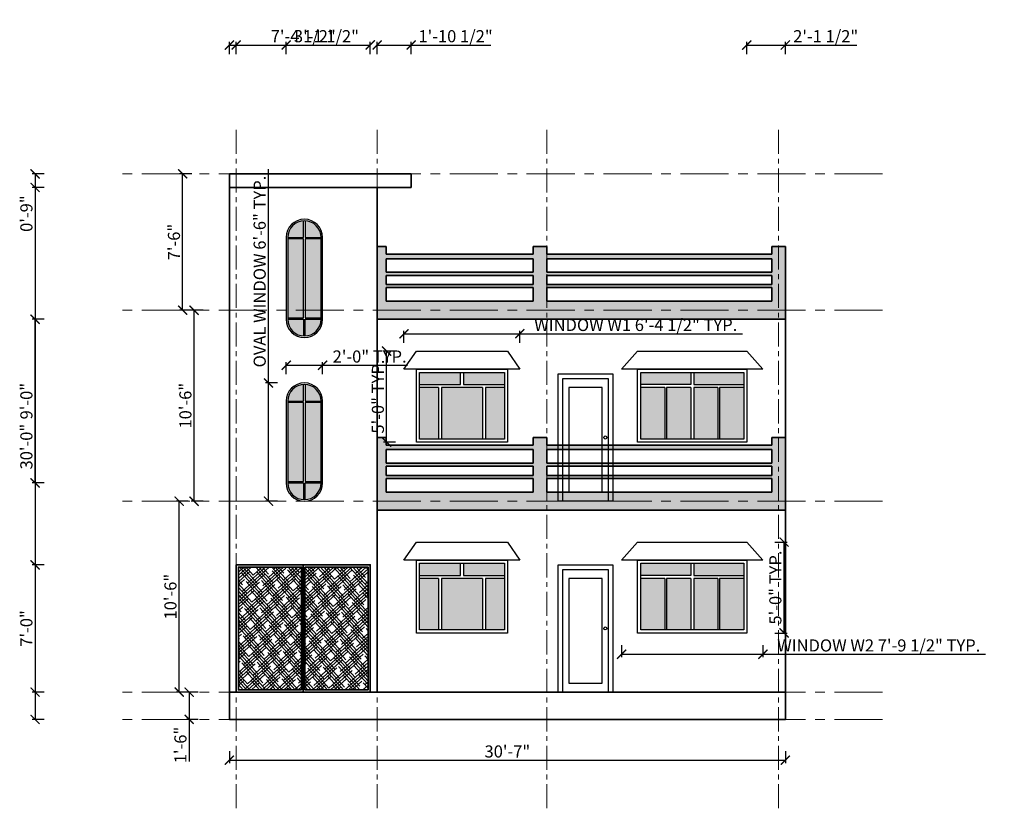
# Model space of a CAD drawing. Units: inches. Extents: x 378 to 1617, y 130 to 1256.
# Tile 3 of 5: x 378 to 1028, y 731 to 1256. Entities that reach past the tile are written whole.
import ezdxf

# ---------------------------------------------------------------- set-up
doc = ezdxf.new("R2010")
doc.units = ezdxf.units.IN
doc.linetypes.add('CENTER', pattern=[50.8, 31.75, -6.35, 6.35, -6.35])
for name, color, linetype, lineweight in [('A-ELEV', 7, 'Continuous', 35), ('A-ELEV-PATT', 8, 'Continuous', 13), ('Dimensions', 153, 'Continuous', 18), ('Doors', 2, 'Continuous', 25), ('Grid lines', 7, 'CENTER', 18), ('Windows', 140, 'Continuous', 25)]:
    doc.layers.add(name, color=color, linetype=linetype, lineweight=lineweight)
doc.styles.get("Standard").update_dxf_attribs({"font": 'arial.ttf'})
doc.dimstyles.new('ISO-25', dxfattribs={"dimtxt": 8, "dimasz": 6, "dimexe": 2, "dimexo": 4, "dimtad": 1, "dimdec": 0, "dimlunit": 3, "dimtxsty": 'Standard', "dimblk": 'ARCHTICK', "dimcen": 2.5, "dimadec": 0, "dimazin": 0, "dimtfac": 1, "dimtdec": 0, "dimtmove": 0, "dimatfit": 3, "dimfxl": 6, "dimfxlon": 1, "dimarcsym": 0})

# ---------------------------------------------------------------- blocks, each defined once
blk = doc.blocks.new('*U17')
blk.add_lwpolyline([(3.12, 0.01), (0.12, 0.01), (0.12, 84.01), (36.12, 84.01), (36.12, 0.01), (33.12, 0.01)])
for points in [[(33.12, 80.99), (33.12, 0.01), (3.12, 0.01), (3.12, 80.99)], [(29.12, 6.01), (29.12, 74.99), (7.12, 74.99), (7.12, 6.01)]]:
    blk.add_lwpolyline(points, close=True)
blk.add_circle((31.12, 42.01), 1)
blk = doc.blocks.new('_ArchTick')
at = {"color": 0, "linetype": 'ByBlock', "const_width": 0.15}
blk.add_lwpolyline([(-0.5, -0.5), (0.5, 0.5)], dxfattribs=at)
blk = doc.blocks.new('*D18')
at = {"layer": 'Defpoints', "color": 0, "transparency": 16777216}
for p in [(516.53, 812.08), (489.95, 794.08), (516.53, 794.08)]:
    blk.add_point(p, dxfattribs=at)
at = {"layer": 'Dimensions', "color": 0, "lineweight": -2, "transparency": 16777216}
for p, q in [((495.95, 812.08), (487.95, 812.08)), ((489.95, 812.08), (489.95, 794.08)), ((495.95, 794.08), (487.95, 794.08)), ((489.95, 794.08), (489.95, 766.32))]:
    blk.add_line(p, q, dxfattribs=at)
at = {"layer": 'Dimensions', "color": 0, "lineweight": -2, "transparency": 16777216, "xscale": 6, "yscale": 6, "zscale": 6}
for p, rotation in [((489.95, 812.08), 90), ((489.95, 794.08), 270)]:
    blk.add_blockref('_ArchTick', p, dxfattribs=dict(at, rotation=rotation))
at = {"layer": 'Dimensions', "color": 0, "transparency": 16777216, "insert": (485.24, 777.2), "char_height": 8, "attachment_point": 5, "rotation": 90}
blk.add_mtext('1\'-6"', dxfattribs=at)
blk = doc.blocks.new('*D19')
at = {"layer": 'Defpoints', "color": 0, "transparency": 16777216}
for p in [(483.37, 938.08), (516.53, 938.08), (516.53, 812.08)]:
    blk.add_point(p, dxfattribs=at)
at = {"layer": 'Dimensions', "color": 0, "lineweight": -2, "transparency": 16777216}
for p, q in [((489.37, 938.08), (481.37, 938.08)), ((483.37, 812.08), (483.37, 938.08)), ((489.37, 812.08), (481.37, 812.08))]:
    blk.add_line(p, q, dxfattribs=at)
at = {"layer": 'Dimensions', "color": 0, "lineweight": -2, "transparency": 16777216, "xscale": 6, "yscale": 6, "zscale": 6}
for p, rotation in [((483.37, 938.08), 90), ((483.37, 812.08), 270)]:
    blk.add_blockref('_ArchTick', p, dxfattribs=dict(at, rotation=rotation))
at = {"layer": 'Dimensions', "color": 0, "transparency": 16777216, "insert": (478.66, 875.08), "char_height": 8, "attachment_point": 5, "rotation": 90}
blk.add_mtext('10\'-6"', dxfattribs=at)
blk = doc.blocks.new('*D20')
at = {"layer": 'Defpoints', "color": 0, "transparency": 16777216}
for p in [(493.24, 1064.08), (516.53, 1064.08), (516.53, 938.08)]:
    blk.add_point(p, dxfattribs=at)
at = {"layer": 'Dimensions', "color": 0, "lineweight": -2, "transparency": 16777216}
for p, q in [((499.24, 1064.08), (491.24, 1064.08)), ((493.24, 938.08), (493.24, 1064.08)), ((499.24, 938.08), (491.24, 938.08))]:
    blk.add_line(p, q, dxfattribs=at)
at = {"layer": 'Dimensions', "color": 0, "lineweight": -2, "transparency": 16777216, "xscale": 6, "yscale": 6, "zscale": 6}
for p, rotation in [((493.24, 1064.08), 90), ((493.24, 938.08), 270)]:
    blk.add_blockref('_ArchTick', p, dxfattribs=dict(at, rotation=rotation))
at = {"layer": 'Dimensions', "color": 0, "transparency": 16777216, "insert": (488.53, 1001.08), "char_height": 8, "attachment_point": 5, "rotation": 90}
blk.add_mtext('10\'-6"', dxfattribs=at)
blk = doc.blocks.new('*D21')
at = {"layer": 'Defpoints', "color": 0, "transparency": 16777216}
for p in [(485.68, 1154.08), (516.53, 1154.08), (516.53, 1064.08)]:
    blk.add_point(p, dxfattribs=at)
at = {"layer": 'Dimensions', "color": 0, "lineweight": -2, "transparency": 16777216}
for p, q in [((491.68, 1154.08), (483.68, 1154.08)), ((485.68, 1064.08), (485.68, 1154.08)), ((491.68, 1064.08), (483.68, 1064.08))]:
    blk.add_line(p, q, dxfattribs=at)
at = {"layer": 'Dimensions', "color": 0, "lineweight": -2, "transparency": 16777216, "xscale": 6, "yscale": 6, "zscale": 6}
for p, rotation in [((485.68, 1154.08), 90), ((485.68, 1064.08), 270)]:
    blk.add_blockref('_ArchTick', p, dxfattribs=dict(at, rotation=rotation))
at = {"layer": 'Dimensions', "color": 0, "transparency": 16777216, "insert": (480.97, 1109.08), "char_height": 8, "attachment_point": 5, "rotation": 90}
blk.add_mtext('7\'-6"', dxfattribs=at)
blk = doc.blocks.new('*D22')
at = {"layer": 'Defpoints', "color": 0, "transparency": 16777216}
for p in [(516.53, 794.08), (883.53, 794.08), (883.53, 767.17)]:
    blk.add_point(p, dxfattribs=at)
at = {"layer": 'Dimensions', "color": 0, "lineweight": -2, "transparency": 16777216}
for p, q in [((516.53, 773.17), (516.53, 765.17)), ((516.53, 767.17), (883.53, 767.17)), ((883.53, 773.17), (883.53, 765.17))]:
    blk.add_line(p, q, dxfattribs=at)
at = {"layer": 'Dimensions', "color": 0, "lineweight": -2, "transparency": 16777216, "xscale": 6, "yscale": 6, "zscale": 6, "rotation": 180}
blk.add_blockref('_ArchTick', (516.53, 767.17), dxfattribs=at)
at = {"layer": 'Dimensions', "color": 0, "lineweight": -2, "transparency": 16777216, "xscale": 6, "yscale": 6, "zscale": 6}
blk.add_blockref('_ArchTick', (883.53, 767.17), dxfattribs=at)
at = {"layer": 'Dimensions', "color": 0, "transparency": 16777216, "insert": (700.03, 771.88), "char_height": 8, "attachment_point": 5}
blk.add_mtext('30\'-7"', dxfattribs=at)
blk = doc.blocks.new('WIN-ELEV-SMALL')
for p, q in [((654.53, 887.08), (654.53, 853.08)), ((656.53, 887.08), (656.53, 853.08)), ((683.53, 887.08), (683.53, 853.08)), ((685.53, 887.08), (685.53, 853.08))]:
    blk.add_line(p, q)
for points in [[(700.03, 911.08), (708.29, 899.08), (631.77, 899.08), (640.03, 911.08)], [(640.03, 851.08), (640.03, 899.08), (700.03, 899.08), (700.03, 851.08)], [(642.03, 853.08), (642.03, 897.08), (698.03, 897.08), (698.03, 853.08)]]:
    blk.add_lwpolyline(points, close=True)
for points in [[(642.03, 889.08), (669.03, 889.08), (669.03, 897.08)], [(671.03, 897.08), (671.03, 889.08), (698.03, 889.08)], [(654.53, 887.08), (642.03, 887.08)], [(683.53, 887.08), (670.03, 887.08), (656.53, 887.08)], [(698.03, 887.08), (685.53, 887.08)]]:
    blk.add_lwpolyline(points)
blk = doc.blocks.new('WIN-ELEV-LARGE')
for p, q in [((821.03, 897.08), (821.03, 889.08)), ((823.03, 897.08), (823.03, 889.08)), ((804.03, 887.08), (804.03, 853.08)), ((805.03, 887.08), (805.03, 853.08)), ((821.03, 887.08), (821.03, 853.08)), ((823.03, 887.08), (823.03, 853.08)), ((839.03, 887.08), (839.03, 853.08)), ((840.03, 887.08), (840.03, 853.08))]:
    blk.add_line(p, q)
for points in [[(775.37, 899.08), (786.03, 911.08), (858.03, 911.08), (868.69, 899.08)], [(786.03, 851.08), (786.03, 899.08), (858.03, 899.08), (858.03, 851.08)], [(788.03, 853.08), (788.03, 897.08), (856.03, 897.08), (856.03, 853.08)]]:
    blk.add_lwpolyline(points, close=True)
for points in [[(821.03, 889.08), (788.03, 889.08)], [(804.03, 887.08), (788.03, 887.08)], [(821.03, 887.08), (805.03, 887.08)], [(823.03, 889.08), (856.03, 889.08)], [(839.03, 887.08), (823.03, 887.08)], [(856.03, 887.08), (840.03, 887.08)]]:
    blk.add_lwpolyline(points)
blk = doc.blocks.new('WIN-ELEV-OVAL')
for points in [[(578.03, 1004.08, 1), (554.03, 1004.08), (554.03, 950.08, 1), (578.03, 950.08)], [(577.03, 1004.08, 1), (555.03, 1004.08), (555.03, 950.08, 1), (577.03, 950.08)]]:
    blk.add_lwpolyline(points, format="xyb", close=True)
for points in [[(555.03, 1004.08), (565.53, 1004.08), (565.53, 1015.08)], [(566.53, 1015.08), (566.53, 1004.08), (577.03, 1004.08)], [(555.03, 951.08), (565.53, 951.08), (565.53, 1003.08), (555.03, 1003.08)], [(577.03, 1003.08), (566.53, 1003.08), (566.53, 951.08), (577.03, 951.08)], [(555.03, 950.08), (565.53, 950.08), (565.53, 939.08)], [(566.53, 939.08), (566.53, 950.08), (577.03, 950.08)]]:
    blk.add_lwpolyline(points)
blk = doc.blocks.new('*D47')
at = {"layer": 'Defpoints', "color": 0, "transparency": 16777216}
for p in [(708.29, 1048.56), (631.77, 1037.08), (708.29, 1037.08)]:
    blk.add_point(p, dxfattribs=at)
at = {"layer": 'Dimensions', "color": 0, "lineweight": -2, "transparency": 16777216}
for p, q in [((631.77, 1042.56), (631.77, 1050.56)), ((631.77, 1048.56), (708.29, 1048.56)), ((708.29, 1042.56), (708.29, 1050.56)), ((708.29, 1048.56), (855.28, 1048.56))]:
    blk.add_line(p, q, dxfattribs=at)
at = {"layer": 'Dimensions', "color": 0, "lineweight": -2, "transparency": 16777216, "xscale": 6, "yscale": 6, "zscale": 6, "rotation": 180}
blk.add_blockref('_ArchTick', (631.77, 1048.56), dxfattribs=at)
at = {"layer": 'Dimensions', "color": 0, "lineweight": -2, "transparency": 16777216, "xscale": 6, "yscale": 6, "zscale": 6}
blk.add_blockref('_ArchTick', (708.29, 1048.56), dxfattribs=at)
at = {"layer": 'Dimensions', "color": 0, "transparency": 16777216, "insert": (784.78, 1053.32), "char_height": 8, "attachment_point": 5}
blk.add_mtext('WINDOW W1 6\'-4 1/2" TYP.', dxfattribs=at)
blk = doc.blocks.new('*D48')
at = {"layer": 'Defpoints', "color": 0, "transparency": 16777216}
for p in [(620.29, 1037.08), (631.77, 1037.08), (631.77, 977.08)]:
    blk.add_point(p, dxfattribs=at)
at = {"layer": 'Dimensions', "color": 0, "lineweight": -2, "transparency": 16777216}
for p, q in [((626.29, 1037.08), (618.29, 1037.08)), ((620.29, 977.08), (620.29, 1037.08)), ((626.29, 977.08), (618.29, 977.08))]:
    blk.add_line(p, q, dxfattribs=at)
at = {"layer": 'Dimensions', "color": 0, "lineweight": -2, "transparency": 16777216, "xscale": 6, "yscale": 6, "zscale": 6}
for p, rotation in [((620.29, 1037.08), 90), ((620.29, 977.08), 270)]:
    blk.add_blockref('_ArchTick', p, dxfattribs=dict(at, rotation=rotation))
at = {"layer": 'Dimensions', "color": 0, "transparency": 16777216, "insert": (615.58, 1007.08), "char_height": 8, "attachment_point": 5, "rotation": 90}
blk.add_mtext('5\'-0" TYP.', dxfattribs=at)
blk = doc.blocks.new('*D49')
at = {"layer": 'Defpoints', "color": 0, "transparency": 16777216}
for p in [(775.37, 851.08), (868.69, 851.08), (868.69, 837.08)]:
    blk.add_point(p, dxfattribs=at)
at = {"layer": 'Dimensions', "color": 0, "lineweight": -2, "transparency": 16777216}
for p, q in [((775.37, 843.08), (775.37, 835.08)), ((868.69, 843.08), (868.69, 835.08)), ((775.37, 837.08), (868.69, 837.08)), ((868.69, 837.08), (1015.68, 837.08))]:
    blk.add_line(p, q, dxfattribs=at)
at = {"layer": 'Dimensions', "color": 0, "lineweight": -2, "transparency": 16777216, "xscale": 6, "yscale": 6, "zscale": 6, "rotation": 180}
blk.add_blockref('_ArchTick', (775.37, 837.08), dxfattribs=at)
at = {"layer": 'Dimensions', "color": 0, "lineweight": -2, "transparency": 16777216, "xscale": 6, "yscale": 6, "zscale": 6}
blk.add_blockref('_ArchTick', (868.69, 837.08), dxfattribs=at)
at = {"layer": 'Dimensions', "color": 0, "transparency": 16777216, "insert": (945.18, 841.85), "char_height": 8, "attachment_point": 5}
blk.add_mtext('WINDOW W2 7\'-9 1/2" TYP.', dxfattribs=at)
blk = doc.blocks.new('*D50')
at = {"layer": 'Defpoints', "color": 0, "transparency": 16777216}
for p in [(868.69, 911.08), (882.68, 911.08), (868.69, 851.08)]:
    blk.add_point(p, dxfattribs=at)
at = {"layer": 'Dimensions', "color": 0, "lineweight": -2, "transparency": 16777216}
for p, q in [((876.68, 911.08), (884.68, 911.08)), ((882.68, 851.08), (882.68, 911.08)), ((876.68, 851.08), (884.68, 851.08))]:
    blk.add_line(p, q, dxfattribs=at)
at = {"layer": 'Dimensions', "color": 0, "lineweight": -2, "transparency": 16777216, "xscale": 6, "yscale": 6, "zscale": 6}
for p, rotation in [((882.68, 911.08), 90), ((882.68, 851.08), 270)]:
    blk.add_blockref('_ArchTick', p, dxfattribs=dict(at, rotation=rotation))
at = {"layer": 'Dimensions', "color": 0, "transparency": 16777216, "insert": (877.97, 881.08), "char_height": 8, "attachment_point": 5, "rotation": 90}
blk.add_mtext('5\'-0" TYP.', dxfattribs=at)
blk = doc.blocks.new('*D51')
at = {"layer": 'Defpoints', "color": 0, "transparency": 16777216}
for p in [(542.33, 1016.08), (554.03, 1016.08), (554.03, 938.08)]:
    blk.add_point(p, dxfattribs=at)
at = {"layer": 'Dimensions', "color": 0, "lineweight": -2, "transparency": 16777216}
for p, q in [((542.33, 1016.08), (542.33, 1157.08)), ((548.33, 1016.08), (540.33, 1016.08)), ((542.33, 938.08), (542.33, 1016.08)), ((548.33, 938.08), (540.33, 938.08))]:
    blk.add_line(p, q, dxfattribs=at)
at = {"layer": 'Dimensions', "color": 0, "lineweight": -2, "transparency": 16777216, "xscale": 6, "yscale": 6, "zscale": 6}
for p, rotation in [((542.33, 1016.08), 90), ((542.33, 938.08), 270)]:
    blk.add_blockref('_ArchTick', p, dxfattribs=dict(at, rotation=rotation))
at = {"layer": 'Dimensions', "color": 0, "transparency": 16777216, "insert": (537.56, 1089.58), "char_height": 8, "attachment_point": 5, "rotation": 90}
blk.add_mtext('OVAL WINDOW 6\'-6" TYP.', dxfattribs=at)
blk = doc.blocks.new('*D52')
at = {"layer": 'Defpoints', "color": 0, "transparency": 16777216}
for p in [(578.03, 1027.78), (554.03, 1016.08), (578.03, 1016.08)]:
    blk.add_point(p, dxfattribs=at)
at = {"layer": 'Dimensions', "color": 0, "lineweight": -2, "transparency": 16777216}
for p, q in [((554.03, 1021.78), (554.03, 1029.78)), ((554.03, 1027.78), (578.03, 1027.78)), ((578.03, 1021.78), (578.03, 1029.78)), ((578.03, 1027.78), (634.18, 1027.78))]:
    blk.add_line(p, q, dxfattribs=at)
at = {"layer": 'Dimensions', "color": 0, "lineweight": -2, "transparency": 16777216, "xscale": 6, "yscale": 6, "zscale": 6, "rotation": 180}
blk.add_blockref('_ArchTick', (554.03, 1027.78), dxfattribs=at)
at = {"layer": 'Dimensions', "color": 0, "lineweight": -2, "transparency": 16777216, "xscale": 6, "yscale": 6, "zscale": 6}
blk.add_blockref('_ArchTick', (578.03, 1027.78), dxfattribs=at)
at = {"layer": 'Dimensions', "color": 0, "transparency": 16777216, "insert": (609.1, 1032.49), "char_height": 8, "attachment_point": 5}
blk.add_mtext('2\'-0" TYP.', dxfattribs=at)
blk = doc.blocks.new('*D74')
at = {"layer": 'Defpoints', "color": 0, "transparency": 16777216}
for p in [(516.53, 1154.08), (388.27, 794.08), (516.53, 794.08)]:
    blk.add_point(p, dxfattribs=at)
at = {"layer": 'Dimensions', "color": 0, "lineweight": -2, "transparency": 16777216}
for p, q in [((394.27, 1154.08), (386.27, 1154.08)), ((388.27, 1154.08), (388.27, 794.08)), ((394.27, 794.08), (386.27, 794.08))]:
    blk.add_line(p, q, dxfattribs=at)
at = {"layer": 'Dimensions', "color": 0, "lineweight": -2, "transparency": 16777216, "xscale": 6, "yscale": 6, "zscale": 6}
for p, rotation in [((388.27, 1154.08), 90), ((388.27, 794.08), 270)]:
    blk.add_blockref('_ArchTick', p, dxfattribs=dict(at, rotation=rotation))
at = {"layer": 'Dimensions', "color": 0, "transparency": 16777216, "insert": (383.55, 974.08), "char_height": 8, "attachment_point": 5, "rotation": 90}
blk.add_mtext('30\'-0"', dxfattribs=at)
blk = doc.blocks.new('*D75')
at = {"layer": 'Defpoints', "color": 0, "transparency": 16777216}
for p in [(636.53, 1239.08), (614.03, 1145.08), (636.53, 1145.08)]:
    blk.add_point(p, dxfattribs=at)
at = {"layer": 'Dimensions', "color": 0, "lineweight": -2, "transparency": 16777216}
for p, q in [((614.03, 1233.08), (614.03, 1241.08)), ((614.03, 1239.08), (636.53, 1239.08)), ((636.53, 1233.08), (636.53, 1241.08)), ((636.53, 1239.08), (689.15, 1239.08))]:
    blk.add_line(p, q, dxfattribs=at)
at = {"layer": 'Dimensions', "color": 0, "lineweight": -2, "transparency": 16777216, "xscale": 6, "yscale": 6, "zscale": 6, "rotation": 180}
blk.add_blockref('_ArchTick', (614.03, 1239.08), dxfattribs=at)
at = {"layer": 'Dimensions', "color": 0, "lineweight": -2, "transparency": 16777216, "xscale": 6, "yscale": 6, "zscale": 6}
blk.add_blockref('_ArchTick', (636.53, 1239.08), dxfattribs=at)
at = {"layer": 'Dimensions', "color": 0, "transparency": 16777216, "insert": (665.84, 1243.84), "char_height": 8, "attachment_point": 5}
blk.add_mtext('1\'-10 1/2"', dxfattribs=at)
blk = doc.blocks.new('*D76')
at = {"layer": 'Defpoints', "color": 0, "transparency": 16777216}
for p in [(883.53, 1106.08), (883.53, 1058.08), (1613.65, 1058.08)]:
    blk.add_point(p, dxfattribs=at)
at = {"layer": 'Dimensions', "color": 0, "lineweight": -2, "transparency": 16777216}
for p, q in [((1607.65, 1106.08), (1615.65, 1106.08)), ((1613.65, 1106.08), (1613.65, 1058.08)), ((1607.65, 1058.08), (1615.65, 1058.08))]:
    blk.add_line(p, q, dxfattribs=at)
at = {"layer": 'Dimensions', "color": 0, "lineweight": -2, "transparency": 16777216, "xscale": 6, "yscale": 6, "zscale": 6}
for p, rotation in [((1613.65, 1106.08), 90), ((1613.65, 1058.08), 270)]:
    blk.add_blockref('_ArchTick', p, dxfattribs=dict(at, rotation=rotation))
at = {"layer": 'Dimensions', "color": 0, "transparency": 16777216, "insert": (1608.94, 1082.08), "char_height": 8, "attachment_point": 5, "rotation": 90}
blk.add_mtext('4\'-0"', dxfattribs=at)
blk = doc.blocks.new('*D77')
at = {"layer": 'Defpoints', "color": 0, "transparency": 16777216}
for p in [(733.65, 812.09), (769.65, 812.09), (769.65, 678.08)]:
    blk.add_point(p, dxfattribs=at)
at = {"layer": 'Dimensions', "color": 0, "lineweight": -2, "transparency": 16777216}
for p, q in [((733.65, 684.08), (733.65, 676.08)), ((769.65, 684.08), (769.65, 676.08)), ((733.65, 678.08), (769.65, 678.08))]:
    blk.add_line(p, q, dxfattribs=at)
at = {"layer": 'Dimensions', "color": 0, "lineweight": -2, "transparency": 16777216, "xscale": 6, "yscale": 6, "zscale": 6, "rotation": 180}
blk.add_blockref('_ArchTick', (733.65, 678.08), dxfattribs=at)
at = {"layer": 'Dimensions', "color": 0, "lineweight": -2, "transparency": 16777216, "xscale": 6, "yscale": 6, "zscale": 6}
blk.add_blockref('_ArchTick', (769.65, 678.08), dxfattribs=at)
at = {"layer": 'Dimensions', "color": 0, "transparency": 16777216, "insert": (751.65, 682.79), "char_height": 8, "attachment_point": 5}
blk.add_mtext('3\'-0"', dxfattribs=at)
blk = doc.blocks.new('*D78')
at = {"layer": 'Defpoints', "color": 0, "transparency": 16777216}
for p in [(733.65, 896.09), (388.27, 812.09), (733.65, 812.09)]:
    blk.add_point(p, dxfattribs=at)
at = {"layer": 'Dimensions', "color": 0, "lineweight": -2, "transparency": 16777216}
for p, q in [((394.27, 896.09), (386.27, 896.09)), ((388.27, 896.09), (388.27, 812.09)), ((394.27, 812.09), (386.27, 812.09))]:
    blk.add_line(p, q, dxfattribs=at)
at = {"layer": 'Dimensions', "color": 0, "lineweight": -2, "transparency": 16777216, "xscale": 6, "yscale": 6, "zscale": 6}
for p, rotation in [((388.27, 896.09), 90), ((388.27, 812.09), 270)]:
    blk.add_blockref('_ArchTick', p, dxfattribs=dict(at, rotation=rotation))
at = {"layer": 'Dimensions', "color": 0, "transparency": 16777216, "insert": (383.56, 854.09), "char_height": 8, "attachment_point": 5, "rotation": 90}
blk.add_mtext('7\'-0"', dxfattribs=at)
blk = doc.blocks.new('*D79')
at = {"layer": 'Defpoints', "color": 0, "transparency": 16777216}
for p in [(609.53, 1239.08), (521.03, 896.08), (609.53, 896.08)]:
    blk.add_point(p, dxfattribs=at)
at = {"layer": 'Dimensions', "color": 0, "lineweight": -2, "transparency": 16777216}
for p, q in [((521.03, 1233.08), (521.03, 1241.08)), ((521.03, 1239.08), (609.53, 1239.08)), ((609.53, 1233.08), (609.53, 1241.08))]:
    blk.add_line(p, q, dxfattribs=at)
at = {"layer": 'Dimensions', "color": 0, "lineweight": -2, "transparency": 16777216, "xscale": 6, "yscale": 6, "zscale": 6, "rotation": 180}
blk.add_blockref('_ArchTick', (521.03, 1239.08), dxfattribs=at)
at = {"layer": 'Dimensions', "color": 0, "lineweight": -2, "transparency": 16777216, "xscale": 6, "yscale": 6, "zscale": 6}
blk.add_blockref('_ArchTick', (609.53, 1239.08), dxfattribs=at)
at = {"layer": 'Dimensions', "color": 0, "transparency": 16777216, "insert": (565.28, 1243.84), "char_height": 8, "attachment_point": 5}
blk.add_mtext('7\'-4 1/2"', dxfattribs=at)
blk = doc.blocks.new('*D80')
at = {"layer": 'Defpoints', "color": 0, "transparency": 16777216}
for p in [(521.03, 896.08), (388.27, 812.08), (521.03, 812.08)]:
    blk.add_point(p, dxfattribs=at)
at = {"layer": 'Dimensions', "color": 0, "lineweight": -2, "transparency": 16777216}
for p, q in [((394.27, 896.08), (386.27, 896.08)), ((388.27, 896.08), (388.27, 812.08)), ((394.27, 812.08), (386.27, 812.08))]:
    blk.add_line(p, q, dxfattribs=at)
at = {"layer": 'Dimensions', "color": 0, "lineweight": -2, "transparency": 16777216, "xscale": 6, "yscale": 6, "zscale": 6}
for p, rotation in [((388.27, 896.08), 90), ((388.27, 812.08), 270)]:
    blk.add_blockref('_ArchTick', p, dxfattribs=dict(at, rotation=rotation))
at = {"layer": 'Dimensions', "color": 0, "transparency": 16777216, "insert": (383.56, 854.08), "char_height": 8, "attachment_point": 5, "rotation": 90}
blk.add_mtext('7\'-0"', dxfattribs=at)
blk = doc.blocks.new('*D81')
at = {"layer": 'Defpoints', "color": 0, "transparency": 16777216}
for p in [(640.03, 851.08), (614.03, 812.08), (640.03, 678.08)]:
    blk.add_point(p, dxfattribs=at)
at = {"layer": 'Dimensions', "color": 0, "lineweight": -2, "transparency": 16777216}
for p, q in [((614.03, 684.08), (614.03, 676.08)), ((640.03, 684.08), (640.03, 676.08)), ((614.03, 678.08), (640.03, 678.08))]:
    blk.add_line(p, q, dxfattribs=at)
at = {"layer": 'Dimensions', "color": 0, "lineweight": -2, "transparency": 16777216, "xscale": 6, "yscale": 6, "zscale": 6, "rotation": 180}
blk.add_blockref('_ArchTick', (614.03, 678.08), dxfattribs=at)
at = {"layer": 'Dimensions', "color": 0, "lineweight": -2, "transparency": 16777216, "xscale": 6, "yscale": 6, "zscale": 6}
blk.add_blockref('_ArchTick', (640.03, 678.08), dxfattribs=at)
at = {"layer": 'Dimensions', "color": 0, "transparency": 16777216, "insert": (627.03, 682.72), "char_height": 8, "attachment_point": 5}
blk.add_mtext('2\'-2"', dxfattribs=at)
blk = doc.blocks.new('*D82')
at = {"layer": 'Defpoints', "color": 0, "transparency": 16777216}
for p in [(700.03, 851.08), (733.65, 812.09), (733.65, 678.08)]:
    blk.add_point(p, dxfattribs=at)
at = {"layer": 'Dimensions', "color": 0, "lineweight": -2, "transparency": 16777216}
for p, q in [((700.03, 684.08), (700.03, 676.08)), ((733.65, 684.08), (733.65, 676.08)), ((700.03, 678.08), (733.65, 678.08)), ((733.65, 678.08), (780.95, 678.08))]:
    blk.add_line(p, q, dxfattribs=at)
at = {"layer": 'Dimensions', "color": 0, "lineweight": -2, "transparency": 16777216, "xscale": 6, "yscale": 6, "zscale": 6, "rotation": 180}
blk.add_blockref('_ArchTick', (700.03, 678.08), dxfattribs=at)
at = {"layer": 'Dimensions', "color": 0, "lineweight": -2, "transparency": 16777216, "xscale": 6, "yscale": 6, "zscale": 6}
blk.add_blockref('_ArchTick', (733.65, 678.08), dxfattribs=at)
at = {"layer": 'Dimensions', "color": 0, "transparency": 16777216, "insert": (760.3, 682.84), "char_height": 8, "attachment_point": 5}
blk.add_mtext('2\'-9 1/2"', dxfattribs=at)
blk = doc.blocks.new('*D83')
at = {"layer": 'Defpoints', "color": 0, "transparency": 16777216}
for p in [(883.53, 1239.08), (858.03, 851.08), (883.53, 812.08)]:
    blk.add_point(p, dxfattribs=at)
at = {"layer": 'Dimensions', "color": 0, "lineweight": -2, "transparency": 16777216}
for p, q in [((858.03, 1233.08), (858.03, 1241.08)), ((858.03, 1239.08), (883.53, 1239.08)), ((883.53, 1233.08), (883.53, 1241.08)), ((883.53, 1239.08), (930.82, 1239.08))]:
    blk.add_line(p, q, dxfattribs=at)
at = {"layer": 'Dimensions', "color": 0, "lineweight": -2, "transparency": 16777216, "xscale": 6, "yscale": 6, "zscale": 6, "rotation": 180}
blk.add_blockref('_ArchTick', (858.03, 1239.08), dxfattribs=at)
at = {"layer": 'Dimensions', "color": 0, "lineweight": -2, "transparency": 16777216, "xscale": 6, "yscale": 6, "zscale": 6}
blk.add_blockref('_ArchTick', (883.53, 1239.08), dxfattribs=at)
at = {"layer": 'Dimensions', "color": 0, "transparency": 16777216, "insert": (910.17, 1243.84), "char_height": 8, "attachment_point": 5}
blk.add_mtext('2\'-1 1/2"', dxfattribs=at)
blk = doc.blocks.new('*D84')
at = {"layer": 'Defpoints', "color": 0, "transparency": 16777216}
for p in [(858.03, 851.08), (883.53, 812.08), (1613.65, 812.08)]:
    blk.add_point(p, dxfattribs=at)
at = {"layer": 'Dimensions', "color": 0, "lineweight": -2, "transparency": 16777216}
for p, q in [((1607.65, 851.08), (1615.65, 851.08)), ((1613.65, 851.08), (1613.65, 812.08)), ((1607.65, 812.08), (1615.65, 812.08))]:
    blk.add_line(p, q, dxfattribs=at)
at = {"layer": 'Dimensions', "color": 0, "lineweight": -2, "transparency": 16777216, "xscale": 6, "yscale": 6, "zscale": 6}
for p, rotation in [((1613.65, 851.08), 90), ((1613.65, 812.08), 270)]:
    blk.add_blockref('_ArchTick', p, dxfattribs=dict(at, rotation=rotation))
at = {"layer": 'Dimensions', "color": 0, "transparency": 16777216, "insert": (1608.94, 831.58), "char_height": 8, "attachment_point": 5, "rotation": 90}
blk.add_mtext('3\'-3"', dxfattribs=at)
blk = doc.blocks.new('*D85')
at = {"layer": 'Defpoints', "color": 0, "transparency": 16777216}
for p in [(554.03, 1239.08), (516.53, 1154.08), (554.03, 1004.08)]:
    blk.add_point(p, dxfattribs=at)
at = {"layer": 'Dimensions', "color": 0, "lineweight": -2, "transparency": 16777216}
for p, q in [((516.53, 1233.08), (516.53, 1241.08)), ((516.53, 1239.08), (554.03, 1239.08)), ((554.03, 1233.08), (554.03, 1241.08)), ((554.03, 1239.08), (601.18, 1239.08))]:
    blk.add_line(p, q, dxfattribs=at)
at = {"layer": 'Dimensions', "color": 0, "lineweight": -2, "transparency": 16777216, "xscale": 6, "yscale": 6, "zscale": 6, "rotation": 180}
blk.add_blockref('_ArchTick', (516.53, 1239.08), dxfattribs=at)
at = {"layer": 'Dimensions', "color": 0, "lineweight": -2, "transparency": 16777216, "xscale": 6, "yscale": 6, "zscale": 6}
blk.add_blockref('_ArchTick', (554.03, 1239.08), dxfattribs=at)
at = {"layer": 'Dimensions', "color": 0, "transparency": 16777216, "insert": (580.6, 1243.85), "char_height": 8, "attachment_point": 5}
blk.add_mtext('3\'-1 1/2"', dxfattribs=at)
blk = doc.blocks.new('*D86')
at = {"layer": 'Defpoints', "color": 0, "transparency": 16777216}
for p in [(388.27, 1058.08), (554.03, 1058.08), (554.03, 950.08)]:
    blk.add_point(p, dxfattribs=at)
at = {"layer": 'Dimensions', "color": 0, "lineweight": -2, "transparency": 16777216}
for p, q in [((394.27, 1058.08), (386.27, 1058.08)), ((388.27, 950.08), (388.27, 1058.08)), ((394.27, 950.08), (386.27, 950.08))]:
    blk.add_line(p, q, dxfattribs=at)
at = {"layer": 'Dimensions', "color": 0, "lineweight": -2, "transparency": 16777216, "xscale": 6, "yscale": 6, "zscale": 6}
for p, rotation in [((388.27, 1058.08), 90), ((388.27, 950.08), 270)]:
    blk.add_blockref('_ArchTick', p, dxfattribs=dict(at, rotation=rotation))
at = {"layer": 'Dimensions', "color": 0, "transparency": 16777216, "insert": (383.56, 1004.08), "char_height": 8, "attachment_point": 5, "rotation": 90}
blk.add_mtext('9\'-0"', dxfattribs=at)
blk = doc.blocks.new('*D93')
at = {"layer": 'Defpoints', "color": 0, "transparency": 16777216}
for p in [(1243.23, 1154.08), (388.27, 1145.08), (1243.23, 1145.08)]:
    blk.add_point(p, dxfattribs=at)
at = {"layer": 'Dimensions', "color": 0, "lineweight": -2, "transparency": 16777216}
for p, q in [((394.27, 1154.08), (386.27, 1154.08)), ((388.27, 1154.08), (388.27, 1145.08)), ((394.27, 1145.08), (386.27, 1145.08)), ((388.27, 1145.08), (388.27, 1116.57))]:
    blk.add_line(p, q, dxfattribs=at)
at = {"layer": 'Dimensions', "color": 0, "lineweight": -2, "transparency": 16777216, "xscale": 6, "yscale": 6, "zscale": 6}
for p, rotation in [((388.27, 1154.08), 90), ((388.27, 1145.08), 270)]:
    blk.add_blockref('_ArchTick', p, dxfattribs=dict(at, rotation=rotation))
at = {"layer": 'Dimensions', "color": 0, "transparency": 16777216, "insert": (383.56, 1127.82), "char_height": 8, "attachment_point": 5, "rotation": 90}
blk.add_mtext('0\'-9"', dxfattribs=at)

msp = doc.modelspace()

# ---------------------------------------------------------------- hatches: boundary and pattern name
at = {"layer": 'A-ELEV-PATT'}
h = msp.add_hatch(dxfattribs=at)
h.set_pattern_fill('GOST_GLASS', color=256, scale=0.8)
h.paths.add_polyline_path([(565.53, 1003.08), (555.03, 1003.08), (555.03, 951.08), (565.53, 951.08)])
h.paths.add_polyline_path([(577.03, 1003.08), (566.53, 1003.08), (566.53, 951.08), (577.03, 951.08)])
h.paths.add_polyline_path([(566.53, 1015.07), (566.53, 1004.08), (577.03, 1004.08, 0.400957)])
h.paths.add_polyline_path([(565.53, 1015.07, 0.400957), (555.03, 1004.08), (565.53, 1004.08)])
h.paths.add_polyline_path([(565.53, 950.08), (555.03, 950.08, 0.400957), (565.53, 939.09)])
h.paths.add_polyline_path([(577.03, 950.08), (566.53, 950.08), (566.53, 939.09, 0.400957)])
h.paths.add_polyline_path([(577.03, 1111.08), (566.53, 1111.08), (566.53, 1059.08), (577.03, 1059.08)])
h.paths.add_polyline_path([(565.53, 1111.08), (555.03, 1111.08), (555.03, 1059.08), (565.53, 1059.08)])
h.paths.add_polyline_path([(565.53, 1058.08), (555.03, 1058.08, 0.400957), (565.53, 1047.09)])
h.paths.add_polyline_path([(577.03, 1058.08), (566.53, 1058.08), (566.53, 1047.09, 0.400957)])
h.paths.add_polyline_path([(566.53, 1123.07), (566.53, 1112.08), (577.03, 1112.08, 0.400957)])
h.paths.add_polyline_path([(565.53, 1123.07, 0.400957), (555.03, 1112.08), (565.53, 1112.08)])
h.paths.add_polyline_path([(683.53, 1013.08), (670.03, 1013.08), (656.53, 1013.08), (656.53, 979.08), (683.53, 979.08)])
h.paths.add_polyline_path([(654.53, 1013.08), (642.03, 1013.08), (642.03, 979.08), (654.53, 979.08)])
h.paths.add_polyline_path([(669.03, 1023.08), (642.03, 1023.08), (642.03, 1015.08), (669.03, 1015.08)])
h.paths.add_polyline_path([(698.03, 1013.08), (685.53, 1013.08), (685.53, 979.08), (698.03, 979.08)])
h.paths.add_polyline_path([(698.03, 1023.08), (671.03, 1023.08), (671.03, 1015.08), (698.03, 1015.08)])
h.paths.add_polyline_path([(804.03, 1013.08), (788.03, 1013.08), (788.03, 979.08), (804.03, 979.08)])
h.paths.add_polyline_path([(821.03, 1013.08), (805.03, 1013.08), (805.03, 979.08), (821.03, 979.08)])
h.paths.add_polyline_path([(821.03, 1023.08), (788.03, 1023.08), (788.03, 1015.08), (821.03, 1015.08)])
h.paths.add_polyline_path([(839.03, 1013.08), (823.03, 1013.08), (823.03, 979.08), (839.03, 979.08)])
h.paths.add_polyline_path([(856.03, 1013.08), (840.03, 1013.08), (840.03, 979.08), (856.03, 979.08)])
h.paths.add_polyline_path([(856.03, 1023.08), (823.03, 1023.08), (823.03, 1015.08), (856.03, 1015.08)])
h.paths.add_polyline_path([(683.53, 887.08), (670.03, 887.08), (656.53, 887.08), (656.53, 853.08), (683.53, 853.08)])
h.paths.add_polyline_path([(654.53, 887.08), (642.03, 887.08), (642.03, 853.08), (654.53, 853.08)])
h.paths.add_polyline_path([(698.03, 887.08), (685.53, 887.08), (685.53, 853.08), (698.03, 853.08)])
h.paths.add_polyline_path([(698.03, 897.08), (671.03, 897.08), (671.03, 889.08), (698.03, 889.08)])
h.paths.add_polyline_path([(669.03, 897.08), (642.03, 897.08), (642.03, 889.08), (669.03, 889.08)])
h.paths.add_polyline_path([(804.03, 887.08), (788.03, 887.08), (788.03, 853.08), (804.03, 853.08)])
h.paths.add_polyline_path([(821.03, 887.08), (805.03, 887.08), (805.03, 853.08), (821.03, 853.08)])
h.paths.add_polyline_path([(839.03, 887.08), (823.03, 887.08), (823.03, 853.08), (839.03, 853.08)])
h.paths.add_polyline_path([(856.03, 887.08), (840.03, 887.08), (840.03, 853.08), (856.03, 853.08)])
h.paths.add_polyline_path([(856.03, 897.08), (823.03, 897.08), (823.03, 889.08), (856.03, 889.08)])
h.paths.add_polyline_path([(821.03, 897.08), (788.03, 897.08), (788.03, 889.08), (821.03, 889.08)])
h.paths.add_polyline_path([(1460.23, 1016.08), (1459.23, 1016.08), (1459.23, 938.08), (1460.23, 938.08)])
h.paths.add_polyline_path([(1460.23, 1124.08), (1459.23, 1124.08), (1459.23, 1046.08), (1460.23, 1046.08)])
h = msp.add_hatch(color=256, dxfattribs=at)
h.dxf.hatch_style = 1
h.paths.add_polyline_path([(883.53, 980.08), (874.53, 980.08), (874.53, 975.08), (726.03, 975.08), (726.03, 980.08), (717.03, 980.08), (717.03, 975.08), (620.03, 975.08), (620.03, 980.08), (614.03, 980.08), (614.03, 932.08), (883.53, 932.08)])
h.paths.add_polyline_path([(620.03, 944.08), (620.03, 953.08), (717.03, 953.08), (717.03, 944.08)], flags=16)
h.paths.add_polyline_path([(620.03, 955.08), (620.03, 961.08), (717.03, 961.08), (717.03, 955.08)], flags=16)
h.paths.add_polyline_path([(620.03, 963.08), (620.03, 972.08), (717.03, 972.08), (717.03, 963.08)], flags=16)
h.paths.add_polyline_path([(726.03, 944.08), (726.03, 953.08), (874.53, 953.08), (874.53, 944.08)], flags=16)
h.paths.add_polyline_path([(726.03, 955.08), (726.03, 961.08), (874.53, 961.08), (874.53, 955.08)], flags=16)
h.paths.add_polyline_path([(726.03, 963.08), (726.03, 972.08), (874.53, 972.08), (874.53, 963.08)], flags=16)
h.paths.add_polyline_path([(883.53, 1106.08), (874.53, 1106.08), (874.53, 1101.08), (726.03, 1101.08), (726.03, 1106.08), (717.03, 1106.08), (717.03, 1101.08), (620.03, 1101.08), (620.03, 1106.08), (614.03, 1106.08), (614.03, 1058.08), (883.53, 1058.08)])
h.paths.add_polyline_path([(717.03, 1070.08), (620.03, 1070.08), (620.03, 1079.08), (717.03, 1079.08)], flags=16)
h.paths.add_polyline_path([(726.03, 1070.08), (726.03, 1079.08), (874.53, 1079.08), (874.53, 1070.08)], flags=16)
h.paths.add_polyline_path([(717.03, 1081.08), (620.03, 1081.08), (620.03, 1087.08), (717.03, 1087.08)], flags=16)
h.paths.add_polyline_path([(726.03, 1081.08), (726.03, 1087.08), (874.53, 1087.08), (874.53, 1081.08)], flags=16)
h.paths.add_polyline_path([(717.03, 1089.08), (620.03, 1089.08), (620.03, 1098.08), (717.03, 1098.08)], flags=16)
h.paths.add_polyline_path([(726.03, 1089.08), (726.03, 1098.08), (874.53, 1098.08), (874.53, 1089.08)], flags=16)
h = msp.add_hatch(dxfattribs=at)
h.set_pattern_fill('HOUND', color=256, angle=42)
h.paths.add_polyline_path([(564.23, 894.58), (522.53, 894.58), (522.53, 813.58), (564.23, 813.58)])
h.paths.add_polyline_path([(608.03, 894.58), (566.33, 894.58), (566.33, 813.58), (608.03, 813.58)])

# ---------------------------------------------------------------- linework, layer by layer
at = {"layer": 'A-ELEV'}
for p, q in [((516.53, 812.08), (516.53, 1154.08)), ((516.53, 1154.08), (636.53, 1154.08)), ((636.53, 1154.08), (636.53, 1145.08)), ((516.53, 1145.08), (636.53, 1145.08)), ((614.03, 1145.08), (614.03, 812.08)), ((614.03, 1058.08), (614.03, 1106.08)), ((614.03, 1106.08), (620.03, 1106.08)), ((620.03, 1101.08), (620.03, 1106.08)), ((717.03, 1101.08), (717.03, 1106.08)), ((717.03, 1106.08), (726.03, 1106.08)), ((726.03, 1101.08), (726.03, 1106.08)), ((874.53, 1101.08), (874.53, 1106.08)), ((874.53, 1106.08), (883.53, 1106.08)), ((883.53, 1058.08), (883.53, 1106.08)), ((620.03, 1101.08), (717.03, 1101.08)), ((726.03, 1101.08), (874.53, 1101.08)), ((620.03, 1098.08), (717.03, 1098.08)), ((620.03, 1089.08), (620.03, 1098.08)), ((717.03, 1089.08), (717.03, 1098.08)), ((726.03, 1098.08), (874.53, 1098.08)), ((726.03, 1089.08), (726.03, 1098.08)), ((874.53, 1089.08), (874.53, 1098.08)), ((620.03, 1089.08), (717.03, 1089.08)), ((620.03, 1087.08), (717.03, 1087.08)), ((620.03, 1081.08), (620.03, 1087.08)), ((717.03, 1081.08), (717.03, 1087.08)), ((726.03, 1089.08), (874.53, 1089.08)), ((726.03, 1087.08), (874.53, 1087.08)), ((726.03, 1081.08), (726.03, 1087.08)), ((874.53, 1081.08), (874.53, 1087.08)), ((620.03, 1081.08), (717.03, 1081.08)), ((620.03, 1079.08), (717.03, 1079.08)), ((620.03, 1070.08), (620.03, 1079.08)), ((717.03, 1070.08), (717.03, 1079.08)), ((726.03, 1081.08), (874.53, 1081.08)), ((726.03, 1079.08), (874.53, 1079.08)), ((726.03, 1070.08), (726.03, 1079.08)), ((874.53, 1070.08), (874.53, 1079.08)), ((620.03, 1070.08), (717.03, 1070.08)), ((726.03, 1070.08), (874.53, 1070.08)), ((614.03, 1058.08), (883.53, 1058.08)), ((883.53, 812.08), (883.53, 1058.08)), ((614.03, 932.08), (614.03, 980.08)), ((614.03, 980.08), (620.03, 980.08)), ((620.03, 975.08), (620.03, 980.08)), ((620.03, 975.08), (717.03, 975.08)), ((717.03, 980.08), (726.03, 980.08)), ((717.03, 975.08), (717.03, 980.08)), ((726.03, 975.08), (726.03, 980.08)), ((726.03, 975.08), (874.53, 975.08)), ((874.53, 980.08), (883.53, 980.08)), ((874.53, 975.08), (874.53, 980.08)), ((883.53, 932.08), (883.53, 980.08)), ((620.03, 972.08), (717.03, 972.08)), ((620.03, 963.08), (620.03, 972.08)), ((717.03, 963.08), (717.03, 972.08)), ((726.03, 972.08), (874.53, 972.08)), ((726.03, 963.08), (726.03, 972.08)), ((874.53, 963.08), (874.53, 972.08)), ((620.03, 963.08), (717.03, 963.08)), ((726.03, 963.08), (874.53, 963.08)), ((620.03, 961.08), (717.03, 961.08)), ((620.03, 955.08), (620.03, 961.08)), ((717.03, 955.08), (717.03, 961.08)), ((726.03, 961.08), (874.53, 961.08)), ((726.03, 955.08), (726.03, 961.08)), ((874.53, 955.08), (874.53, 961.08)), ((620.03, 955.08), (717.03, 955.08)), ((620.03, 944.08), (620.03, 953.08)), ((620.03, 953.08), (717.03, 953.08)), ((717.03, 944.08), (717.03, 953.08)), ((726.03, 955.08), (874.53, 955.08)), ((726.03, 944.08), (726.03, 953.08)), ((726.03, 953.08), (874.53, 953.08)), ((874.53, 944.08), (874.53, 953.08)), ((620.03, 944.08), (717.03, 944.08)), ((726.03, 944.08), (874.53, 944.08)), ((614.03, 932.08), (883.53, 932.08)), ((516.53, 812.08), (516.53, 794.08)), ((516.53, 812.08), (883.53, 812.08)), ((883.53, 812.08), (883.53, 794.08)), ((516.53, 794.08), (883.53, 794.08))]:
    msp.add_line(p, q, dxfattribs=at)
for points in [[(565.23, 812.08), (521.03, 812.08), (521.03, 896.08), (565.23, 896.08)], [(564.23, 813.58), (522.53, 813.58), (522.53, 894.58), (564.23, 894.58)], [(565.33, 896.08), (609.53, 896.08), (609.53, 812.08), (565.33, 812.08)], [(566.33, 894.58), (608.03, 894.58), (608.03, 813.58), (566.33, 813.58)]]:
    msp.add_lwpolyline(points, close=True, dxfattribs=at)
at = {"layer": 'Grid lines', "ltscale": 0.5}
for p, q in [((521.03, 1183.08), (521.03, 734.08)), ((614.03, 1183.08), (614.03, 734.08)), ((726.03, 1183.08), (726.03, 734.08)), ((879.03, 1183.08), (879.03, 734.08))]:
    msp.add_line(p, q, dxfattribs=at)
at = {"layer": 'Grid lines'}
for p, q in [((947.71, 1154.08), (444.27, 1154.08)), ((947.71, 1064.08), (444.27, 1064.08)), ((947.71, 938.08), (444.27, 938.08)), ((947.71, 812.08), (444.27, 812.08)), ((947.71, 794.08), (444.27, 794.08))]:
    msp.add_line(p, q, dxfattribs=at)

# ---------------------------------------------------------------- block references
at = {"layer": 'Doors'}
for p in [(733.53, 938.08), (733.53, 812.08)]:
    msp.add_blockref('*U17', p, dxfattribs=at)
at = {"layer": 'Windows'}
for name, p in [('WIN-ELEV-OVAL', (0, 108)), ('WIN-ELEV-SMALL', (0, 126)), ('WIN-ELEV-LARGE', (0, 126)), ('WIN-ELEV-OVAL', (0, 0)), ('WIN-ELEV-SMALL', (0, 0)), ('WIN-ELEV-LARGE', (0, 0))]:
    msp.add_blockref(name, p, dxfattribs=at)

# ---------------------------------------------------------------- dimensions: what is measured, and where the dimension line sits
at = {"layer": 'Dimensions'}
for base, p1, p2, override, picture, middle in [((554.03, 1239.08), (516.53, 1154.08), (554.03, 1004.08), {"dimdec": 1, "dimlfac": 1, "dimrnd": 0, "dimzin": 1, "dimdsep": 46, "dimlunit": 4, "dimfrac": 2}, '*D85', (580.6, 1243.85)), ((609.53, 1239.08), (521.03, 896.08), (609.53, 896.08), {"dimdec": 1, "dimlfac": 1, "dimrnd": 0, "dimzin": 1, "dimdsep": 46, "dimlunit": 4, "dimfrac": 2}, '*D79', (565.28, 1243.84)), ((636.53, 1239.08), (614.03, 1145.08), (636.53, 1145.08), {"dimdec": 1, "dimlfac": 1, "dimrnd": 0, "dimzin": 1, "dimdsep": 46, "dimlunit": 4, "dimfrac": 2}, '*D75', (665.84, 1243.84)), ((883.53, 1239.08), (858.03, 851.08), (883.53, 812.08), {"dimdec": 1, "dimlfac": 1, "dimrnd": 0, "dimzin": 1, "dimdsep": 46, "dimlunit": 4, "dimfrac": 2}, '*D83', (910.17, 1243.84)), ((640.03, 678.08), (614.03, 812.08), (640.03, 851.08), {"dimdec": 1, "dimlfac": 1, "dimrnd": 0, "dimzin": 1, "dimdsep": 46, "dimlunit": 4, "dimfrac": 2}, '*D81', (627.03, 682.72)), ((733.65, 678.08), (700.03, 851.08), (733.65, 812.09), {"dimdec": 1, "dimlfac": 1, "dimrnd": 0, "dimzin": 1, "dimdsep": 46, "dimlunit": 4, "dimfrac": 2}, '*D82', (760.3, 682.84)), ((769.65, 678.08), (733.65, 812.09), (769.65, 812.09), {"dimdec": 1, "dimlfac": 1, "dimrnd": 0, "dimzin": 1, "dimdsep": 46, "dimlunit": 4, "dimfrac": 2}, '*D77', (751.65, 682.79)), ((883.53, 767.17), (516.53, 794.08), (883.53, 794.08), {"dimclrd": 0, "dimclre": 0, "dimclrt": 0}, '*D22', (700.03, 771.88))]:
    dim = msp.add_linear_dim(base=base, p1=p1, p2=p2, dimstyle='ISO-25', override=override, dxfattribs=at)
    dim.commit()
    dim.dimension.update_dxf_attribs({"geometry": picture, "text_midpoint": middle})
for base, p1, p2, override, picture, middle in [((388.27, 794.08), (516.53, 1154.08), (516.53, 794.08), {"dimdec": 1, "dimlfac": 1, "dimrnd": 0, "dimzin": 1, "dimdsep": 46, "dimlunit": 4, "dimfrac": 2}, '*D74', (383.55, 974.08)), ((388.27, 1145.08), (1243.23, 1154.08), (1243.23, 1145.08), {"dimdec": 1, "dimlfac": 1, "dimrnd": 0, "dimzin": 1, "dimdsep": 46, "dimlunit": 4, "dimfrac": 2}, '*D93', (383.56, 1127.82)), ((485.68, 1154.08), (516.53, 1064.08), (516.53, 1154.08), {"dimclrd": 0, "dimclre": 0, "dimclrt": 0}, '*D21', (480.97, 1109.08)), ((1613.65, 1058.08), (883.53, 1106.08), (883.53, 1058.08), {"dimdec": 1, "dimlfac": 1, "dimrnd": 0, "dimzin": 1, "dimdsep": 46, "dimlunit": 4, "dimfrac": 2}, '*D76', (1608.94, 1082.08)), ((493.24, 1064.08), (516.53, 938.08), (516.53, 1064.08), {"dimclrd": 0, "dimclre": 0, "dimclrt": 0}, '*D20', (488.53, 1001.08)), ((388.27, 1058.08), (554.03, 950.08), (554.03, 1058.08), {"dimdec": 1, "dimlfac": 1, "dimrnd": 0, "dimzin": 1, "dimdsep": 46, "dimlunit": 4, "dimfrac": 2}, '*D86', (383.56, 1004.08)), ((483.37, 938.08), (516.53, 812.08), (516.53, 938.08), {"dimclrd": 0, "dimclre": 0, "dimclrt": 0}, '*D19', (478.66, 875.08)), ((388.27, 812.09), (733.65, 896.09), (733.65, 812.09), {"dimdec": 1, "dimlfac": 1, "dimrnd": 0, "dimzin": 1, "dimdsep": 46, "dimlunit": 4, "dimfrac": 2}, '*D78', (383.56, 854.09)), ((388.27, 812.08), (521.03, 896.08), (521.03, 812.08), {"dimdec": 1, "dimlfac": 1, "dimrnd": 0, "dimzin": 1, "dimdsep": 46, "dimlunit": 4, "dimfrac": 2}, '*D80', (383.56, 854.08)), ((1613.65, 812.08), (858.03, 851.08), (883.53, 812.08), {"dimdec": 1, "dimlfac": 1, "dimrnd": 0, "dimzin": 1, "dimdsep": 46, "dimlunit": 4, "dimfrac": 2}, '*D84', (1608.94, 831.58)), ((489.95, 794.08), (516.53, 812.08), (516.53, 794.08), {"dimclrd": 0, "dimclre": 0, "dimclrt": 0}, '*D18', (485.24, 777.2))]:
    dim = msp.add_linear_dim(base=base, p1=p1, p2=p2, angle=90, dimstyle='ISO-25', override=override, dxfattribs=at)
    dim.commit()
    dim.dimension.update_dxf_attribs({"geometry": picture, "text_midpoint": middle})
for base, p1, p2, text, picture, middle in [((542.33, 1016.08), (554.03, 938.08), (554.03, 1016.08), 'OVAL WINDOW <> TYP.', '*D51', (537.56, 1089.58)), ((620.29, 1037.08), (631.77, 977.08), (631.77, 1037.08), '<> TYP.', '*D48', (615.58, 1007.08)), ((882.68, 911.08), (868.69, 851.08), (868.69, 911.08), '<> TYP.', '*D50', (877.97, 881.08))]:
    dim = msp.add_linear_dim(base=base, p1=p1, p2=p2, angle=90, text=text, dimstyle='ISO-25', override={"dimdec": 1, "dimrnd": 0, "dimzin": 1, "dimlunit": 4, "dimfrac": 2}, dxfattribs=at)
    dim.commit()
    dim.dimension.update_dxf_attribs({"geometry": picture, "text_midpoint": middle})
for base, p1, p2, text, picture, middle in [((708.29, 1048.56), (631.77, 1037.08), (708.29, 1037.08), 'WINDOW W1 <> TYP.', '*D47', (784.78, 1053.32)), ((578.03, 1027.78), (554.03, 1016.08), (578.03, 1016.08), '<> TYP.', '*D52', (609.1, 1032.49)), ((868.69, 837.08), (775.37, 851.08), (868.69, 851.08), 'WINDOW W2 <> TYP.', '*D49', (945.18, 841.85))]:
    dim = msp.add_linear_dim(base=base, p1=p1, p2=p2, text=text, dimstyle='ISO-25', override={"dimdec": 1, "dimrnd": 0, "dimzin": 1, "dimlunit": 4, "dimfrac": 2}, dxfattribs=at)
    dim.commit()
    dim.dimension.update_dxf_attribs({"geometry": picture, "text_midpoint": middle})

doc.saveas('drawing.dxf')
